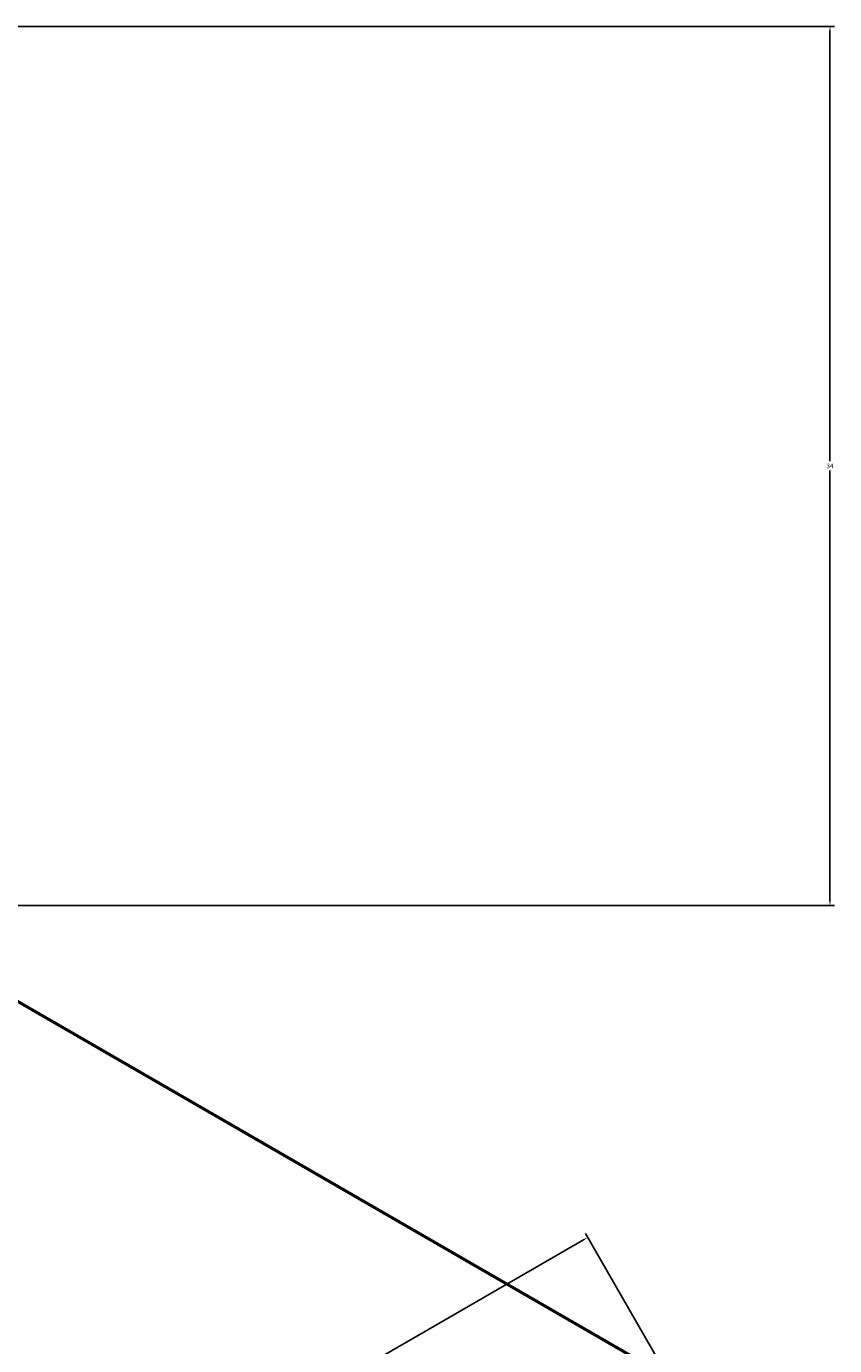
# Model space of a CAD drawing. Units: inches. Extents: x -23 to 69, y -27 to 96.
# Tile 10 of 10: x 37 to 69, y 35 to 86. Entities that reach past the tile are written whole.
import ezdxf

# ---------------------------------------------------------------- set-up
doc = ezdxf.new("R2010")
doc.units = ezdxf.units.IN
doc.header["$MEASUREMENT"] = 0
doc.layers.add('M-DIMS', color=2, linetype='Continuous', lineweight=18)
doc.layers.add('M-OUTL', color=7, linetype='Continuous', lineweight=50)
doc.styles.get("Standard").update_dxf_attribs({"font": 'arial.ttf'})
doc.dimstyles.get("Standard").update_dxf_attribs({"dimtxt": 0.18, "dimasz": 0.18, "dimexe": 0.18, "dimexo": 0.0625, "dimgap": 0.09, "dimtad": 0, "dimtih": 1, "dimtoh": 1, "dimdec": 4, "dimzin": 0, "dimdsep": 46, "dimtxsty": 'Standard', "dimcen": 0.09, "dimadec": 0, "dimazin": 0, "dimtfac": 1, "dimtdec": 4, "dimtofl": 0, "dimtmove": 0, "dimatfit": 3, "dimfxl": 1, "dimtolj": 1, "dimtzin": 0, "dimarcsym": 0})

# ---------------------------------------------------------------- blocks, each defined once
blk = doc.blocks.new('*D1')
at = {"layer": 'Defpoints', "color": 0, "transparency": 16777216}
for p in [(59.046, 39.281), (62.171, 33.869), (16.271, 7.369)]:
    blk.add_point(p, dxfattribs=at)
at = {"layer": 'M-DIMS', "color": 0, "lineweight": -2, "transparency": 16777216}
for p, q in [((62.139, 33.923), (58.956, 39.437)), ((58.89, 39.191), (36.315, 26.158)), ((13.302, 12.871), (35.877, 25.905)), ((16.24, 7.423), (13.056, 12.937))]:
    blk.add_line(p, q, dxfattribs=at)
at = {"layer": 'M-DIMS', "color": 0, "transparency": 16777216}
for points in [[(58.875, 39.217), (58.905, 39.165), (59.046, 39.281)], [(13.287, 12.897), (13.317, 12.845), (13.146, 12.781)]]:
    blk.add_solid(points, dxfattribs=at)
at = {"layer": 'M-DIMS', "color": 0, "transparency": 16777216, "insert": (36.096, 26.031), "char_height": 0.18, "attachment_point": 5}
blk.add_mtext('\\A1;53', dxfattribs=at)
blk = doc.blocks.new('*D15')
at = {"layer": 'Defpoints', "color": 0, "transparency": 16777216}
for p in [(21.034, 86.119), (68.421, 86.119), (17.57, 52.119)]:
    blk.add_point(p, dxfattribs=at)
at = {"layer": 'M-DIMS', "color": 0, "lineweight": -2, "transparency": 16777216}
for p, q in [((21.097, 86.119), (68.601, 86.119)), ((68.421, 85.939), (68.421, 69.301)), ((68.421, 52.299), (68.421, 68.937)), ((17.633, 52.119), (68.601, 52.119))]:
    blk.add_line(p, q, dxfattribs=at)
at = {"layer": 'M-DIMS', "color": 0, "transparency": 16777216}
for points in [[(68.391, 85.939), (68.451, 85.939), (68.421, 86.119)], [(68.391, 52.299), (68.451, 52.299), (68.421, 52.119)]]:
    blk.add_solid(points, dxfattribs=at)
at = {"layer": 'M-DIMS', "color": 0, "transparency": 16777216, "insert": (68.421, 69.119), "char_height": 0.18, "attachment_point": 5}
blk.add_mtext('\\A1;34', dxfattribs=at)

msp = doc.modelspace()

# ---------------------------------------------------------------- linework, layer by layer
at = {"layer": 'M-OUTL'}
msp.add_line((62.1706, 33.8686), (34.4578, 49.8686), dxfattribs=at)

# ---------------------------------------------------------------- dimensions: what is measured, and where the dimension line sits
at = {"layer": 'M-DIMS'}
for base, p1, p2, angle, picture, middle in [((68.4206, 86.1186), (17.5703, 52.1186), (21.0344, 86.1186), 90, '*D15', (68.4206, 69.1186)), ((59.0456, 39.2813), (16.2712, 7.3686), (62.1706, 33.8686), 30, '*D1', (36.0959, 26.0313))]:
    dim = msp.add_linear_dim(base=base, p1=p1, p2=p2, angle=angle, dimstyle='Standard', override={"dimdec": 0, "dimlfac": 1, "dimrnd": 0, "dimzin": 0, "dimdsep": 46, "dimlunit": 2}, dxfattribs=at)
    dim.commit()
    dim.dimension.update_dxf_attribs({"geometry": picture, "text_midpoint": middle})

doc.saveas('drawing.dxf')
